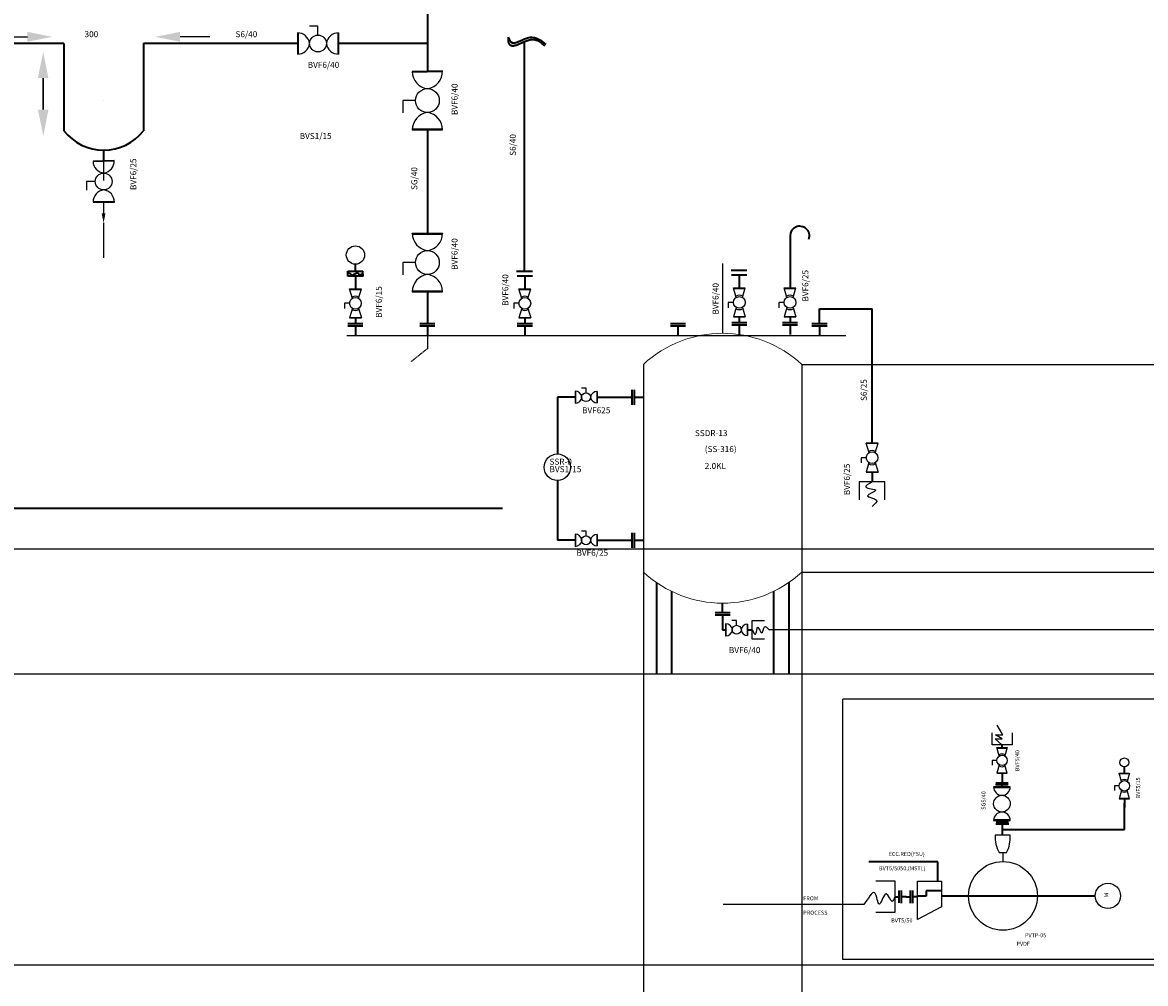
# Model space of a CAD drawing. Units: millimetres. Extents: x 353872 to 441597, y 126154 to 187356.
# Tile 21 of 28: x 399262 to 417572, y 141384 to 157042. Entities that reach past the tile are written whole.
import ezdxf

# ---------------------------------------------------------------- set-up
doc = ezdxf.new("R2010")
doc.units = ezdxf.units.MM
doc.linetypes.add('ACAD_ISO02W100', pattern=[15, 12, -3])
for name, color, linetype, lineweight in [('A-ANNO-DIMS', 2, 'Continuous', 18), ('P-ANNO-TEXT', 7, 'Continuous', 25), ('P-BNDY', 4, 'ACAD_ISO02W100', 25), ('P-INST', 6, 'Continuous', 25), ('P-INST-SIGN', 4, 'Continuous', 18), ('P-PIPE', 3, 'Continuous', 35), ('P-PIPE-FITT', 6, 'Continuous', 25), ('P-SYMB-PATT', 8, 'Continuous', 13), ('P-VALV', 2, 'Continuous', 25)]:
    doc.layers.add(name, color=color, linetype=linetype, lineweight=lineweight)
doc.layers.add('AC-UINT', color=2, linetype='Continuous')
doc.styles.get("Standard").update_dxf_attribs({"font": 'arial.ttf'})
doc.dimstyles.get("Standard").update_dxf_attribs({"dimtxt": 0.18, "dimasz": 0.18, "dimexe": 0.18, "dimexo": 0.0625, "dimgap": 0.09, "dimtad": 0, "dimtih": 1, "dimtoh": 1, "dimdec": 4, "dimzin": 0, "dimdsep": 46, "dimtxsty": 'Standard', "dimcen": 0.09, "dimadec": 0, "dimazin": 0, "dimtfac": 1, "dimtdec": 4, "dimtofl": 0, "dimtmove": 0, "dimatfit": 3, "dimfxl": 1, "dimtolj": 1, "dimtzin": 0, "dimarcsym": 0})

# ---------------------------------------------------------------- blocks, each defined once
blk = doc.blocks.new('DFSG')
at = {"layer": 'AC-UINT', "ltscale": 3}
blk.add_line((94.3237, -27.1601), (94.091, -27.1601), dxfattribs=at)
blk.add_solid([(94.091, -27.1214), (94.0909, -27.1989), (93.8965, -27.1598)], dxfattribs=at)
blk = doc.blocks.new('VALVE-B')
for points in [[(0, 12), (347, 12)], [(0, 8), (347, 8)], [(0, 4), (0, 0), (347, 0), (347, 5)], [(0, 4), (0, 4), (343, 4), (347, 4)]]:
    blk.add_lwpolyline(points)
for centre, radius, start, end in [((199, 2), 199, 97.3612, 180.5798), ((149, 3), 198, 359.2193, 82.8397)]:
    blk.add_arc(centre, radius, start, end)
blk = doc.blocks.new('VALVE-E')
for points in [[(0, 7), (197, 7)], [(0, 5), (197, 4)], [(0, 2), (0, 0), (197, 0), (197, 3)], [(0, 2), (0, 2), (195, 2), (197, 2)]]:
    blk.add_lwpolyline(points)
for centre, start, end in [((113, 1), 97.3612, 180.5798), ((85, 2), 359.2193, 82.8397)]:
    blk.add_arc(centre, 113, start, end)
blk = doc.blocks.new('VALVE-G')
for p, q in [((46, 155), (0, 0)), ((0, 0), (194, 0)), ((2, 7), (192, 7)), ((147, 155), (194, 0))]:
    blk.add_line(p, q)
blk = doc.blocks.new('VALVE-H-INDICATOR')
for points in [[(246, 185), (246, 0)], [(248, 185), (248, 0)], [(250, 185), (252, 185), (252, 0), (250, 0)], [(250, 185), (250, 183), (250, 2), (250, 0)]]:
    blk.add_lwpolyline(points)
blk.add_circle((73, 93), 73)
for centre, start, end in [((251, 79), 89.4202, 172.6388), ((251, 106), 187.1603, 270.7807)]:
    blk.add_arc(centre, 106, start, end)
blk = doc.blocks.new('VALVE-J')
for points in [[(0, 17), (494, 17)], [(0, 11), (494, 11)], [(0, 6), (0, 0), (494, 0), (494, 8)], [(0, 6), (0, 6), (488, 6), (494, 6)]]:
    blk.add_lwpolyline(points)
for centre, radius, start, end in [((283, 3), 283, 97.3612, 180.5798), ((212, 4), 282, 359.2193, 82.8397)]:
    blk.add_arc(centre, radius, start, end)
blk = doc.blocks.new('VALVE-M')
for p, q in [((46, 0), (0, 155)), ((0, 155), (194, 155)), ((147, 0), (194, 155))]:
    blk.add_line(p, q)
blk = doc.blocks.new('*D30')
at = {"layer": 'A-ANNO-DIMS', "color": 0, "lineweight": -2, "transparency": 16777216}
for p, q in [((396728, 148465), (440591, 148465)), ((440591, 148464), (440591, 145075)), ((440591, 141686), (440591, 145075)), ((396728, 141686), (440591, 141686))]:
    blk.add_line(p, q, dxfattribs=at)
at = {"layer": 'A-ANNO-DIMS', "color": 0, "transparency": 16777216}
for points in [[(440591, 148464), (440591, 148464), (440591, 148465)], [(440591, 141686), (440591, 141686), (440591, 141686)]]:
    blk.add_solid(points, dxfattribs=at)
at = {"layer": 'Defpoints', "color": 0, "transparency": 16777216}
for p in [(396728, 148465), (396728, 141686), (440591, 141686)]:
    blk.add_point(p, dxfattribs=at)
at = {"layer": 'A-ANNO-DIMS', "color": 0, "transparency": 16777216, "insert": (440591, 145075), "char_height": 0.18, "attachment_point": 5}
blk.add_mtext('\\A1;6779', dxfattribs=at)
blk = doc.blocks.new('*D31')
at = {"layer": 'A-ANNO-DIMS', "color": 0, "lineweight": -2, "transparency": 16777216}
for p, q in [((409385, 151471), (409385, 133813)), ((411968, 151471), (411968, 133813)), ((409385, 133813), (410676, 133813)), ((411967, 133813), (410677, 133813))]:
    blk.add_line(p, q, dxfattribs=at)
at = {"layer": 'A-ANNO-DIMS', "color": 0, "transparency": 16777216}
for points in [[(409385, 133813), (409385, 133813), (409385, 133813)], [(411967, 133813), (411967, 133813), (411968, 133813)]]:
    blk.add_solid(points, dxfattribs=at)
at = {"layer": 'Defpoints', "color": 0, "transparency": 16777216}
for p in [(409385, 151471), (411968, 151471), (411968, 133813)]:
    blk.add_point(p, dxfattribs=at)
at = {"layer": 'A-ANNO-DIMS', "color": 0, "transparency": 16777216, "insert": (410676, 133813), "char_height": 0.18, "attachment_point": 5}
blk.add_mtext('\\A1;2583', dxfattribs=at)
blk = doc.blocks.new('*D32')
at = {"layer": 'A-ANNO-DIMS', "color": 0, "lineweight": -2, "transparency": 16777216}
for p, q in [((411968, 151471), (440591, 151471)), ((440591, 151471), (440591, 149780)), ((440591, 148088), (440591, 149779)), ((411968, 148088), (440591, 148088))]:
    blk.add_line(p, q, dxfattribs=at)
at = {"layer": 'A-ANNO-DIMS', "color": 0, "transparency": 16777216}
for points in [[(440591, 151471), (440591, 151471), (440591, 151471)], [(440591, 148088), (440591, 148088), (440591, 148088)]]:
    blk.add_solid(points, dxfattribs=at)
at = {"layer": 'Defpoints', "color": 0, "transparency": 16777216}
for p in [(411968, 151471), (411968, 148088), (440591, 148088)]:
    blk.add_point(p, dxfattribs=at)
at = {"layer": 'A-ANNO-DIMS', "color": 0, "transparency": 16777216, "insert": (440591, 149780), "char_height": 0.18, "attachment_point": 5}
blk.add_mtext('\\A1;3383', dxfattribs=at)
blk = doc.blocks.new('*D40')
at = {"layer": 'A-ANNO-DIMS', "color": 0, "lineweight": -2, "transparency": 16777216}
for p, q in [((410676, 153117), (410676, 153117)), ((410676, 153117), (410676, 151978)), ((410676, 150079), (410676, 150079)), ((410676, 150079), (410676, 150079))]:
    blk.add_line(p, q, dxfattribs=at)
at = {"layer": 'A-ANNO-DIMS', "color": 0, "transparency": 16777216}
blk.add_solid([(410676, 151978), (410676, 151978), (410676, 151978)], dxfattribs=at)
at = {"layer": 'Defpoints', "color": 0, "transparency": 16777216}
for p in [(410676, 151978), (410676, 150079)]:
    blk.add_point(p, dxfattribs=at)
at = {"layer": 'A-ANNO-DIMS', "color": 0, "transparency": 16777216, "insert": (410675, 153117), "char_height": 0.18, "attachment_point": 5}
blk.add_mtext('\\A1;2X R1899', dxfattribs=at)
blk = doc.blocks.new('*D41')
at = {"layer": 'A-ANNO-DIMS', "color": 0, "lineweight": -2, "transparency": 16777216}
for p, q in [((400586, 155779), (400587, 155779)), ((400586, 155779), (400586, 155779)), ((400586, 154469), (400586, 154960)), ((400586, 154469), (400586, 154469))]:
    blk.add_line(p, q, dxfattribs=at)
at = {"layer": 'A-ANNO-DIMS', "color": 0, "transparency": 16777216}
blk.add_solid([(400586, 154960), (400586, 154960), (400586, 154961)], dxfattribs=at)
at = {"layer": 'Defpoints', "color": 0, "transparency": 16777216}
for p in [(400586, 155779), (400586, 154961)]:
    blk.add_point(p, dxfattribs=at)
at = {"layer": 'A-ANNO-DIMS', "color": 0, "transparency": 16777216, "insert": (400586, 154469), "char_height": 0.18, "attachment_point": 5}
blk.add_mtext('\\A1;R818.5', dxfattribs=at)

msp = doc.modelspace()

# ---------------------------------------------------------------- hatches: boundary and pattern name
at = {"layer": 'P-SYMB-PATT'}
h = msp.add_hatch(color=256, dxfattribs=at)
h.dxf.hatch_style = 1
edge = h.paths.add_edge_path()
edge.add_spline(control_points=[(407181.27, 156805.44), (407181, 156802.43), (407180.73, 156799.39), (407179.94, 156790.2), (407179.43, 156783.98), (407178.6, 156770.95), (407178.28, 156764.14), (407178.18, 156750.5), (407178.38, 156743.68), (407179.47, 156732.97), (407180, 156729.17), (407181.32, 156722.49), (407182, 156719.63), (407183.71, 156713.83), (407184.71, 156710.95), (407187.86, 156703.42), (407190.31, 156698.83), (407196.27, 156690.17), (407199.78, 156686.11), (407207.63, 156678.98), (407211.94, 156675.9), (407220.88, 156670.92), (407225.49, 156668.99), (407234.62, 156666.12), (407239.15, 156665.17), (407247.99, 156663.96), (407252.32, 156663.71), (407264.45, 156663.68), (407272.04, 156664.49), (407287.07, 156667.08), (407294.51, 156668.87), (407309.5, 156673.15), (407317.05, 156675.64), (407332.35, 156681.14), (407340.11, 156684.15), (407364.7, 156694.13), (407381.93, 156701.76), (407416.88, 156717.24), (407434.59, 156725.09), (407469.52, 156739.56), (407486.74, 156746.17), (407510.86, 156753.97), (407518.44, 156756.18), (407530.99, 156759.35), (407536.1, 156760.49), (407545.08, 156762.19), (407549.01, 156762.82), (407556.77, 156763.82), (407560.58, 156764.2), (407571.82, 156764.97), (407579.06, 156765.01), (407598.47, 156763.98), (407610.28, 156762.06), (407633.45, 156756), (407644.81, 156751.86), (407667.44, 156741.6), (407678.71, 156735.47), (407701.28, 156721.61), (407712.58, 156713.86), (407739.73, 156694.06), (407755.65, 156681.49), (407773.13, 156660.81)], knot_values=[0, 0, 0, 0, 1.45657696, 1.45657696, 4.36973087, 4.36973087, 7.5343006, 7.5343006, 10.69887033, 10.69887033, 12.40671205, 12.40671205, 13.63901259, 13.63901259, 14.87131314, 14.87131314, 16.90061252, 16.90061252, 18.92991189, 18.92991189, 20.95921127, 20.95921127, 22.98851065, 22.98851065, 25.01781003, 25.01781003, 27.04710941, 27.04710941, 30.82532254, 30.82532254, 34.60353567, 34.60353567, 38.38174881, 38.38174881, 42.15996194, 42.15996194, 50.18983557, 50.18983557, 58.21970919, 58.21970919, 66.24958282, 66.24958282, 70.07411996, 70.07411996, 72.8401263, 72.8401263, 75.12034604, 75.12034604, 77.40056578, 77.40056578, 81.96100526, 81.96100526, 89.95516575, 89.95516575, 97.94932623, 97.94932623, 105.94348671, 105.94348671, 113.9376472, 113.9376472, 125.00201057, 125.00201057, 125.00201057, 125.00201057], degree=3, periodic=0)
edge.add_line((407773.13, 156660.81), (407797.09, 156682.59))
edge.add_spline(control_points=[(407797.09, 156682.59), (407716.97, 156749.4), (407620.85, 156829.54), (407496.02, 156792.85), (407475, 156785.08)], knot_values=[65.29657048, 65.29657048, 65.29657048, 65.29657048, 118.21354525, 128.78520648, 128.78520648, 128.78520648, 128.78520648], degree=3, periodic=0)
edge.add_spline(control_points=[(407475, 156785.08), (407377.07, 156748.91), (407240.27, 156653.25), (407192.92, 156775.4), (407181.27, 156805.44)], knot_values=[0, 0, 0, 0, 49.23816608, 65.29657048, 65.29657048, 65.29657048, 65.29657048], degree=3, periodic=0)

# ---------------------------------------------------------------- linework, layer by layer
at = {"layer": 'P-BNDY'}
for p, q in [((400584.23, 153775.23), (400584.23, 153205.34)), ((404550.86, 151943.32), (412684.32, 151943.32)), ((405862.9, 151943.32), (405862.9, 151727.53)), ((405862.9, 151727.53), (405599.59, 151516.9)), ((421575.93, 147147.69), (411431.48, 147147.69)), ((396910.35, 146429.42), (434124.06, 146429.42)), ((412977.03, 142673.32), (410686.77, 142673.32))]:
    msp.add_line(p, q, dxfattribs=at)
msp.add_lwpolyline([(412638.66, 146021.69), (418177.75, 146021.69), (418177.75, 141776.76), (412638.66, 141776.76)], close=True, dxfattribs=at)
at = {"layer": 'P-INST'}
for centre, radius in [((404690.79, 153253.02), 149.4), ((404690.79, 153253.02), 149.4), ((407982.05, 149795.72), 215.85), ((407982.05, 149795.72), 215.85), ((417226.25, 144985.99), 72.34), ((415248.01, 142811.42), 560.73), ((416957.78, 142811.42), 206.04)]:
    msp.add_circle(centre, radius, dxfattribs=at)
at = {"layer": 'P-INST-SIGN'}
for points in [[(409384.78, 151470.92), (409384.78, 148088.1)], [(411967.63, 148088.1), (411967.63, 151470.92)]]:
    msp.add_lwpolyline(points, dxfattribs=at)
for centre, start, end in [((410676.21, 150078.67), 47.151541, 132.848459), ((410676.21, 149480.35), 227.151541, 312.848459)]:
    msp.add_arc(centre, 1898.98, start, end, dxfattribs=at)
at = {"layer": 'P-PIPE'}
for p, q in [((405863.95, 157658.81), (405863.95, 156248.03)), ((399938.88, 156699.54), (398036.88, 156699.54)), ((399938.88, 156699.54), (399938.88, 155278.47)), ((403755.5, 156699.54), (401233.97, 156699.54)), ((401233.97, 156699.54), (401233.97, 155278.47)), ((405863.95, 156699.56), (404416.31, 156699.56)), ((407446.41, 152991.81), (407446.41, 156729.97)), ((405863.95, 155290.92), (405863.95, 153610.33)), ((400586.42, 154788.48), (400586.42, 154960.61)), ((411775.32, 153564.57), (411775.32, 152717.24)), ((405863.95, 153326.52), (405863.95, 153326.43)), ((404690.79, 152991.81), (404690.79, 153104.45)), ((404565.87, 152991.81), (404813.39, 152991.81)), ((404565.87, 152910.79), (404565.87, 152991.81)), ((404815.71, 152910.79), (404565.87, 152910.79)), ((404690.79, 152910.79), (404690.79, 152702.59)), ((404815.71, 152910.79), (404813.39, 152991.81)), ((407318.02, 152991.81), (407574.8, 152991.81)), ((407577.11, 152910.79), (407327.27, 152910.79)), ((407452.19, 152910.79), (407452.19, 152702.59)), ((410814.76, 153006.45), (411071.54, 153006.45)), ((411073.85, 152925.43), (410824.02, 152925.43)), ((410948.94, 152925.43), (410948.94, 152717.24)), ((405863.93, 152653.22), (405863.93, 152309.68)), ((412256.05, 152133.88), (412256.05, 152377.19)), ((412256.05, 152377.19), (413113.91, 152377.19)), ((413113.91, 150187.76), (413113.91, 152377.19)), ((404690.79, 152230.41), (404690.79, 152133.88)), ((404690.92, 152237.63), (404690.92, 152237.46)), ((405863.93, 152309.68), (405863.93, 152133.88)), ((407452.19, 152230.41), (407452.19, 152133.88)), ((407452.32, 152237.63), (407452.32, 152237.46)), ((410948.94, 152245.05), (410948.94, 152148.52)), ((410949.07, 152252.27), (410949.07, 152252.11)), ((411775.32, 152245.05), (411775.32, 152148.52)), ((411775.46, 152252.27), (411775.45, 152252.11)), ((404813.17, 152133.88), (404568.41, 152133.88)), ((404813.17, 152094.72), (404568.41, 152094.72)), ((404690.79, 152094.72), (404690.79, 151943.32)), ((405985.28, 152133.88), (405740.52, 152133.88)), ((405985.28, 152094.72), (405740.52, 152094.72)), ((405862.9, 152094.72), (405862.9, 151943.32)), ((407574.57, 152133.88), (407329.81, 152133.88)), ((407574.57, 152094.72), (407329.81, 152094.72)), ((407452.19, 152094.72), (407452.19, 151943.32)), ((410071.06, 152133.88), (409826.3, 152133.88)), ((410071.06, 152094.72), (409826.3, 152094.72)), ((409948.68, 152094.72), (409948.68, 151943.32)), ((411071.32, 152148.52), (410826.56, 152148.52)), ((411071.32, 152109.37), (410826.56, 152109.37)), ((410948.94, 152109.37), (410948.94, 151957.97)), ((411897.7, 152148.52), (411652.94, 152148.52)), ((411897.7, 152109.37), (411652.94, 152109.37)), ((411775.32, 152109.37), (411775.32, 151957.97)), ((412378.43, 152133.88), (412133.67, 152133.88)), ((412378.43, 152094.72), (412133.67, 152094.72)), ((412256.05, 152094.72), (412256.05, 151943.32)), ((409194.22, 151058.24), (409194.22, 150813.48)), ((409233.38, 151058.24), (409233.38, 150813.48)), ((408271.43, 150936.87), (407982.05, 150936.87)), ((407982.05, 150936.87), (407982.05, 150011.58)), ((408635.92, 150936.88), (409194.22, 150936.88)), ((409233.38, 150935.86), (409384.78, 150935.86)), ((413113.91, 149715.58), (413113.91, 149555.71)), ((407982.05, 149579.87), (407982.05, 148606.25)), ((386450.69, 149129.17), (407087.67, 149129.17)), ((409194.22, 148728.64), (409194.22, 148483.88)), ((409233.38, 148728.64), (409233.38, 148483.88)), ((408271.43, 148606.25), (407982.05, 148606.25)), ((408635.92, 148606.26), (409194.22, 148606.26)), ((409233.38, 148606.26), (409384.78, 148606.26)), ((409596.84, 147917.95), (409596.84, 146429.42)), ((409843.61, 147773.62), (409843.61, 146429.42)), ((411508.8, 147773.62), (411508.8, 146429.42)), ((411755.58, 147917.95), (411755.58, 146429.42)), ((410676.21, 147429.97), (410676.21, 147581.36)), ((410553.83, 147429.97), (410798.59, 147429.97)), ((410553.83, 147390.81), (410798.59, 147390.81)), ((410676.21, 147390.81), (410676.21, 147147.69)), ((410676.21, 147147.69), (410731.36, 147146.64)), ((411083.77, 147146.65), (411155.3, 147146.65)), ((415232.69, 145228.9), (415233.47, 145270.94)), ((417226.25, 144813.86), (417226.25, 144913.65)), ((415130.66, 144651.4), (415333.17, 144651.4)), ((415231.92, 144810.75), (415231.92, 144666.46)), ((415231.92, 144681.52), (415231.92, 144651.4)), ((415334.05, 144620.82), (415125.91, 144620.82)), ((415230.94, 144586.35), (415231.58, 144620.82)), ((417226.25, 144395.71), (417226.25, 144251.42)), ((417226.25, 143891.05), (417226.25, 144322.02)), ((415340.52, 143981.12), (415132.38, 143981.12)), ((415137.13, 144011.7), (415339.64, 144011.7)), ((415241.88, 143800.97), (415238.05, 143981.12)), ((415238.39, 144041.82), (415238.39, 144011.7)), ((415239.96, 143891.05), (417226.25, 143891.05)), ((414186.01, 143364.54), (413061.43, 143364.54)), ((414186.01, 143049.83), (414186.01, 143364.54)), ((413554.95, 142697.06), (413554.95, 142899.57)), ((413585.53, 142900.44), (413585.53, 142692.3)), ((413740.08, 142695.16), (413740.08, 142897.68)), ((413770.66, 142898.55), (413770.66, 142690.41)), ((414245, 142896.39), (413995.59, 142896.39)), ((413995.59, 142896.39), (413995.59, 142809.33)), ((413484.5, 142798.31), (413554.95, 142798.31)), ((413669.63, 142796.42), (413585.53, 142797.97)), ((413669.63, 142796.42), (413740.08, 142796.42)), ((413854.76, 142794.53), (413770.66, 142796.08)), ((413995.59, 142809.33), (413854.76, 142809.33)), ((414245, 142811.42), (416751.74, 142811.42))]:
    msp.add_line(p, q, dxfattribs=at)
for centre, radius, start, end in [((400586.42, 155779.14), 818.53, 217.71019, 322.28981), ((411933.56, 153564.57), 158.24, 340.937078, 180)]:
    msp.add_arc(centre, radius, start, end, dxfattribs=at)
for points, knots in [([(407181.27, 156805.44), (407181, 156802.43), (407180.73, 156799.39), (407179.94, 156790.2), (407179.43, 156783.98), (407178.6, 156770.95), (407178.28, 156764.14), (407178.18, 156750.5), (407178.38, 156743.68), (407179.47, 156732.97), (407180, 156729.17), (407181.32, 156722.49), (407182, 156719.63), (407183.71, 156713.83), (407184.71, 156710.95), (407187.86, 156703.42), (407190.31, 156698.83), (407196.27, 156690.17), (407199.78, 156686.11), (407207.63, 156678.98), (407211.94, 156675.9), (407220.88, 156670.92), (407225.49, 156668.99), (407234.62, 156666.12), (407239.15, 156665.17), (407247.99, 156663.96), (407252.32, 156663.71), (407264.45, 156663.68), (407272.04, 156664.49), (407287.07, 156667.08), (407294.51, 156668.87), (407309.5, 156673.15), (407317.05, 156675.64), (407332.35, 156681.14), (407340.11, 156684.15), (407364.7, 156694.13), (407381.93, 156701.76), (407416.88, 156717.24), (407434.59, 156725.09), (407469.52, 156739.56), (407486.74, 156746.17), (407510.86, 156753.97), (407518.44, 156756.18), (407530.99, 156759.35), (407536.1, 156760.49), (407545.08, 156762.19), (407549.01, 156762.82), (407556.77, 156763.82), (407560.58, 156764.2), (407571.82, 156764.97), (407579.06, 156765.01), (407598.47, 156763.98), (407610.28, 156762.06), (407633.45, 156756), (407644.81, 156751.86), (407667.44, 156741.6), (407678.71, 156735.47), (407701.28, 156721.61), (407712.58, 156713.86), (407739.73, 156694.06), (407755.65, 156681.49), (407773.13, 156660.81)], [0, 0, 0, 0, 1.45657696, 1.45657696, 4.36973087, 4.36973087, 7.5343006, 7.5343006, 10.69887033, 10.69887033, 12.40671205, 12.40671205, 13.63901259, 13.63901259, 14.87131314, 14.87131314, 16.90061252, 16.90061252, 18.92991189, 18.92991189, 20.95921127, 20.95921127, 22.98851065, 22.98851065, 25.01781003, 25.01781003, 27.04710941, 27.04710941, 30.82532254, 30.82532254, 34.60353567, 34.60353567, 38.38174881, 38.38174881, 42.15996194, 42.15996194, 50.18983557, 50.18983557, 58.21970919, 58.21970919, 66.24958282, 66.24958282, 70.07411996, 70.07411996, 72.8401263, 72.8401263, 75.12034604, 75.12034604, 77.40056578, 77.40056578, 81.96100526, 81.96100526, 89.95516575, 89.95516575, 97.94932623, 97.94932623, 105.94348671, 105.94348671, 113.9376472, 113.9376472, 125.00201057, 125.00201057, 125.00201057, 125.00201057]), ([(407181.27, 156805.44), (407192.92, 156775.4), (407247.94, 156633.47), (407546.3, 156891.7), (407716.97, 156749.4), (407797.09, 156682.59)], [0, 0, 0, 0, 86.88313995, 410.4810187, 696.78548649, 696.78548649, 696.78548649, 696.78548649]), ([(404565.87, 152951.3), (404580.61, 152955.13), (404605.3, 152961.56), (404626.93, 152905.71), (404682, 152958.7), (404743.45, 152969.61), (404764.02, 152901.8), (404796.69, 152955.91), (404815.33, 152951.11), (404815.71, 152951.01)], [0, 0, 0, 0, 38.99490026, 65.30631279, 141.03895925, 190.36959254, 226.63856921, 283.00446007, 284.20420132, 284.20420132, 284.20420132, 284.20420132])]:
    msp.add_open_spline(points, degree=3, knots=knots, dxfattribs=at)
at = {"layer": 'P-VALV'}
for p, q in [((410854.89, 152707.76), (411042.98, 152707.76)), ((411681.28, 152707.76), (411869.37, 152707.76)), ((404596.74, 152693.12), (404784.83, 152693.12)), ((407358.15, 152693.12), (407546.24, 152693.12)), ((404595.19, 152466.5), (404511.17, 152466.5)), ((404511.17, 152466.5), (404511.17, 152380.94)), ((407356.59, 152466.5), (407272.58, 152466.5)), ((407272.58, 152466.5), (407272.58, 152380.94)), ((410853.34, 152481.14), (410769.32, 152481.14)), ((410769.32, 152481.14), (410769.32, 152395.58)), ((411679.72, 152481.14), (411595.71, 152481.14)), ((411595.71, 152481.14), (411595.71, 152395.58)), ((413018.31, 149951.67), (412934.3, 149951.67)), ((412934.3, 149951.67), (412934.3, 149866.11)), ((415148.64, 145220.51), (415315.2, 145220.51)), ((415147.99, 144817), (415315.84, 144817)), ((417142.97, 144805.46), (417309.53, 144805.46)), ((417142.33, 144401.96), (417310.18, 144401.96)), ((415362.9, 143800.97), (415120.85, 143800.97)), ((415362.9, 143708.22), (415362.9, 143800.97)), ((415184.43, 143517.83), (415248.01, 143517.83)), ((415248.01, 143372.15), (415248.01, 143517.83)), ((415248.01, 143517.83), (415305.46, 143517.83)), ((413854.76, 142425.08), (413854.76, 143049.83)), ((413854.76, 143049.83), (414245, 143049.83)), ((414245, 143049.83), (414245, 142634.7)), ((414245, 142634.7), (413854.76, 142425.08))]:
    msp.add_line(p, q, dxfattribs=at)
for points in [[(404079.87, 156836.88), (404079.87, 156980.17), (403939.18, 156980.17)], [(404404.28, 156872.95), (404404.19, 156526.14)], [(404408.37, 156873.11), (404408.53, 156525.98)], [(404412.28, 156873.19), (404416.31, 156873.19), (404416.31, 156525.93), (404410.91, 156525.93)], [(404412.47, 156873.19), (404412.42, 156869.3), (404412.42, 156529.83), (404412.39, 156525.92)], [(405668.61, 155769.48), (405464.79, 155769.48), (405464.79, 155569.36)], [(400449.11, 154452.03), (400305.81, 154452.03), (400305.81, 154311.34)], [(405616.96, 153604.6), (405616.96, 153610.33), (406110.9, 153610.33), (406110.9, 153602.64)], [(405616.96, 153604.87), (405622.5, 153604.79), (406105.36, 153604.79), (406110.92, 153604.76)], [(405617.07, 153599.03), (406110.83, 153599.26)], [(405617.3, 153593.22), (406110.6, 153593.09)], [(405668.61, 153131.78), (405464.79, 153131.78), (405464.79, 152931.65)], [(408450.86, 151010.1), (408450.86, 151086.53), (408375.83, 151086.53)], [(413323.93, 149262.43), (413323.93, 149555.71), (412903.89, 149555.71), (412903.89, 149262.43)], [(408450.86, 148679.48), (408450.86, 148755.9), (408375.83, 148755.9)], [(410904.34, 147219.88), (410904.34, 147296.31), (410829.31, 147296.31)], [(411360.59, 147293.66), (411155.3, 147293.66), (411155.3, 146999.65), (411360.59, 146999.65)], [(415228.71, 145270.94), (415121.19, 145369.08), (415233.47, 145369.08), (415124.87, 145434.12), (415246.36, 145434.12), (415154.32, 145592.28)], [(415397.29, 145467.22), (415397.29, 145270.94), (415069.65, 145270.94), (415069.65, 145467.22)], [(415187.29, 145091.76), (415146.12, 145228.9), (415317.72, 145228.9), (415276.55, 145091.76)], [(415147.26, 145019.82), (415072.86, 145019.82), (415072.86, 144944.06)], [(415187.29, 144947.89), (415146.12, 144810.75), (415317.72, 144810.75), (415276.55, 144947.89)], [(417181.62, 144676.72), (417140.45, 144813.86), (417312.05, 144813.86), (417270.88, 144676.72)], [(415366.6, 144573.71), (415095.29, 144573.71)], [(417141.59, 144604.78), (417067.19, 144604.78), (417067.19, 144529.02)], [(417181.62, 144532.85), (417140.45, 144395.71), (417312.05, 144395.71), (417270.88, 144532.85)], [(415095.29, 144054.47), (415366.6, 144054.47)], [(413174.53, 143057.02), (413484.5, 143057.02), (413484.5, 142539.6), (413174.53, 142539.6)]]:
    msp.add_lwpolyline(points, dxfattribs=at)
for points in [[(415367.19, 144586.35), (415094.7, 144586.35, 1)], [(415094.7, 144041.82), (415367.19, 144041.82, 1)]]:
    msp.add_lwpolyline(points, format="xyb", close=True, dxfattribs=at)
for centre, radius in [((404079.87, 156700.02), 136.85), ((405863.27, 155769.48), 194.66), ((400585.96, 154452.03), 136.85), ((405863.27, 153131.78), 194.66), ((404690.79, 152466.5), 95.6), ((407452.19, 152466.5), 95.6), ((410948.94, 152481.14), 95.6), ((411775.32, 152481.14), 95.6), ((413113.91, 149951.67), 95.6), ((415231.92, 145019.82), 84.66), ((417226.25, 144604.78), 84.66), ((415230.94, 144314.09), 136.24)]:
    msp.add_circle(centre, radius, dxfattribs=at)
for centre, radius, start, end in [((404414.3, 156674.05), 199.16, 89.420152, 172.638767), ((404413.61, 156724.29), 198.38, 187.160335, 270.780747), ((405900.22, 153607.46), 283.28, 179.420152, 262.638767), ((405828.76, 153606.49), 282.17, 277.160335, 0.780747), ((404690.79, 152466.5), 117.04, 60.998829, 119.001171), ((407452.19, 152466.5), 117.04, 60.998829, 119.001171), ((410948.94, 152481.14), 117.04, 60.998829, 119.001171), ((411775.32, 152481.14), 117.04, 60.998829, 119.001171), ((404690.79, 152466.5), 117.04, 240.998829, 299.001171), ((407452.19, 152466.5), 117.04, 240.998829, 299.001171), ((410948.94, 152481.14), 117.04, 240.998829, 299.001171), ((411775.32, 152481.14), 117.04, 240.998829, 299.001171), ((413113.91, 149951.67), 117.04, 60.998829, 119.001171), ((413113.91, 149951.67), 117.04, 240.998829, 299.001171), ((415231.92, 145019.82), 103.65, 60.998829, 119.001171), ((415231.92, 145019.82), 103.65, 240.998829, 299.001171), ((417226.25, 144604.78), 103.65, 60.998829, 119.001171), ((417226.25, 144604.78), 103.65, 240.998829, 299.001171), ((415609.75, 143762.05), 490.44, 175.447638, 209.864188), ((414864.98, 143754.6), 500.08, 331.741199, 5.321321)]:
    msp.add_arc(centre, radius, start, end, dxfattribs=at)
for points, knots in [([(413113.91, 149555.71), (413055.45, 149523.25), (412922.21, 149449.29), (413307.8, 149442.34), (412913.92, 149313.45), (413263.89, 149284.41), (413158.68, 149197.08), (413112.5, 149158.75)], [0, 0, 0, 0, 131.62046813, 299.94883433, 460.08690619, 621.6605897, 748.04024912, 748.04024912, 748.04024912, 748.04024912]), ([(411155.3, 147146.65), (411178.02, 147105.73), (411229.79, 147012.47), (411234.66, 147282.36), (411324.87, 147006.67), (411345.2, 147251.63), (411406.33, 147177.99), (411433.16, 147145.67)], [0, 0, 0, 0, 92.12866386, 209.95127675, 322.04103606, 435.13566174, 523.59598502, 523.59598502, 523.59598502, 523.59598502]), ([(413484.5, 142798.31), (413470.9, 142760.41), (413432.95, 142654.64), (413333.37, 142989.32), (413222.57, 142514.9), (413169.83, 143026.98), (413043.99, 142747.38), (412977.03, 142673.32)], [0, 0, 0, 0, 19.81712218, 55.3026495, 100.82402837, 145.47117908, 204.21404416, 204.21404416, 204.21404416, 204.21404416])]:
    msp.add_open_spline(points, degree=3, knots=knots, dxfattribs=at)

# ---------------------------------------------------------------- block references
at = {"layer": 'P-PIPE-FITT'}
for p, xscale, yscale, zscale, rotation in [((595010.25, 100175.78), 2079.990875364621, 2079.990875364621, 2079.990875364621, 179.9589088552121), ((206162.6, 100175.78), -2079.990875364621, 2079.990875364621, 2079.990875364621, 180.0410911447878), ((459671.86, 363688.73), 2206.336445412279, 2206.336445412279, 2206.336445412279, 269.9589088552122), ((459673.04, -51931.33), -2206.336445412279, 2206.336445412278, 2206.336445412278, 270.0410911447879), ((378695.2, 78100.76), 805.9348046081378, 805.9348046081378, 805.9348046081378, 89.99999999999991)]:
    msp.add_blockref('DFSG', p, dxfattribs=dict(at, xscale=xscale, yscale=yscale, zscale=zscale, rotation=rotation))
at = {"layer": 'P-VALV'}
for name, p, rotation in [('VALVE-B', (403743.43, 156873.19), 270.0000000001145), ('VALVE-J', (406109.82, 156253.64), 181.3019170022079), ('VALVE-B', (400759.3, 154792.42), 181.3019170021816), ('VALVE-E', (408270.51, 151035.61), 270.0000000002378), ('VALVE-G', (413210.88, 150186.97), 179.887796659946), ('VALVE-E', (408270.51, 148704.98), 270.0000000002352), ('VALVE-E', (410724, 147245.39), 270.0000000003056)]:
    msp.add_blockref(name, p, dxfattribs=dict(at, rotation=rotation))
for name, p in [('VALVE-J', (405616.96, 155290.92)), ('VALVE-B', (400412.79, 154115.59)), ('VALVE-J', (405616.96, 152653.22)), ('VALVE-M', (410852.05, 152562.38)), ('VALVE-M', (411678.43, 152562.38)), ('VALVE-M', (404593.9, 152547.73)), ('VALVE-M', (407355.3, 152547.73)), ('VALVE-G', (404593.9, 152230.41)), ('VALVE-G', (407355.3, 152230.41)), ('VALVE-G', (410852.05, 152245.05)), ('VALVE-G', (411678.43, 152245.05)), ('VALVE-H-INDICATOR', (408377.88, 150844.27)), ('VALVE-G', (413017.02, 149715.58)), ('VALVE-H-INDICATOR', (408377.88, 148513.64)), ('VALVE-H-INDICATOR', (410831.36, 147054.05))]:
    msp.add_blockref(name, p, dxfattribs=at)

# ---------------------------------------------------------------- texts
at = {"layer": 'P-ANNO-TEXT'}
for s, height, p in [('300', 98.09, (400274.67, 156802.58)), ('S6/40', 98.09, (402735.14, 156802.58)), ('BVF6/40', 98.09, (403912.4, 156302.66)), ('BVS1/15', 98.09, (403781.63, 155143.64)), ('BVF625', 98.09, (408385.17, 150674.98)), ('SSDR-13', 98.09, (410224.59, 150302.95)), ('(SS-316)', 98.09, (410385.65, 150042.63)), ('SSR-0', 98.09, (407854.33, 149837.55)), ('BVS1/15', 98.09, (407854.33, 149715.44)), ('2.0KL', 98.09, (410385.65, 149768.12)), ('BVF6/25', 98.09, (408295.18, 148352.9)), ('BVF6/40', 98.09, (410778.97, 146766.97)), ('ECC.RED(FSU)', 65.2854, (413384.32, 143462.59)), ('BVT5/5050,(MSTL)', 65.2854, (413226.08, 143228.23)), ('FROM', 65.285, (411991.72, 142739.91)), ('PROCESS', 65.285, (411991.72, 142505.54)), ('BVT5/50', 65.285, (413425.56, 142379.27)), ('PVTP-05', 65.285, (415606.67, 142136.93)), ('PVDF', 65.285, (415468.09, 141998.24))]:
    msp.add_text(s, height=height, dxfattribs=at).set_placement(p)
for s, height, p in [('BVF6/40', 98.09, (406355.18, 155533.88)), ('S6/40', 98.09, (407305.58, 154869.35)), ('BVF6/25', 98.09, (401118.07, 154312.92)), ('SG/40', 98.09, (405698.53, 154312.92)), ('BVF6/40', 98.09, (406355.18, 153012.82)), ('BVF6/40', 98.09, (407182.34, 152426.26)), ('BVF6/25', 98.09, (412075.12, 152495.75)), ('BVF6/15', 98.09, (405121.02, 152230.41)), ('BVF6/40', 98.09, (410611.11, 152284.15)), ('S6/25', 98.09, (413027.44, 150875.55)), ('BVF6/25', 98.09, (412751.94, 149339.69)), ('BVF5/40', 65.285, (415512.61, 144845.04)), ('BVF5/15', 65.285, (417483.67, 144400.36)), ('SGS/40', 65.285, (414962.59, 144214.91)), ('M', 65.29, (416966.27, 142788.9))]:
    msp.add_text(s, height=height, rotation=90, dxfattribs=at).set_placement(p)

# ---------------------------------------------------------------- dimensions: what is measured, and where the dimension line sits
at = {"layer": 'A-ANNO-DIMS'}
dim = msp.add_radius_dim(center=(400586.42, 155779.14), mpoint=(400586.4, 154960.61), dimstyle='Standard', override={"dimdec": 1, "dimlfac": 1, "dimrnd": 0, "dimzin": 0, "dimdsep": 46, "dimlunit": 2}, dxfattribs=at)
dim.commit()
dim.dimension.update_dxf_attribs({"geometry": '*D41', "text_midpoint": (400585.72, 154469.49), "dimtype": 164})
dim = msp.add_radius_dim(center=(410676.21, 150078.67), mpoint=(410676.2, 151977.65), text='2X <>', dimstyle='Standard', override={"dimdec": 0, "dimlfac": 1, "dimrnd": 0, "dimzin": 0, "dimdsep": 46, "dimlunit": 2}, dxfattribs=at)
dim.commit()
dim.dimension.update_dxf_attribs({"geometry": '*D40', "text_midpoint": (410675.38, 153117.04), "dimtype": 164})
dim = msp.add_linear_dim(base=(411967.63, 133812.84), p1=(409384.78, 151470.92), p2=(411967.63, 151470.92), dimstyle='Standard', override={"dimdec": 0, "dimlfac": 1, "dimrnd": 0, "dimzin": 0, "dimdsep": 46, "dimlunit": 2}, dxfattribs=at)
dim.commit()
dim.dimension.update_dxf_attribs({"geometry": '*D31', "text_midpoint": (410676.21, 133812.84)})
for base, p1, p2, picture, middle in [((440591, 148088.1), (411967.63, 151470.92), (411967.63, 148088.1), '*D32', (440591, 149779.51)), ((440591, 141685.82), (396727.53, 148464.52), (396727.53, 141685.82), '*D30', (440591, 145075.17))]:
    dim = msp.add_linear_dim(base=base, p1=p1, p2=p2, angle=90, dimstyle='Standard', override={"dimdec": 0, "dimlfac": 1, "dimrnd": 0, "dimzin": 0, "dimdsep": 46, "dimlunit": 2}, dxfattribs=at)
    dim.commit()
    dim.dimension.update_dxf_attribs({"geometry": picture, "text_midpoint": middle})

doc.saveas('drawing.dxf')
